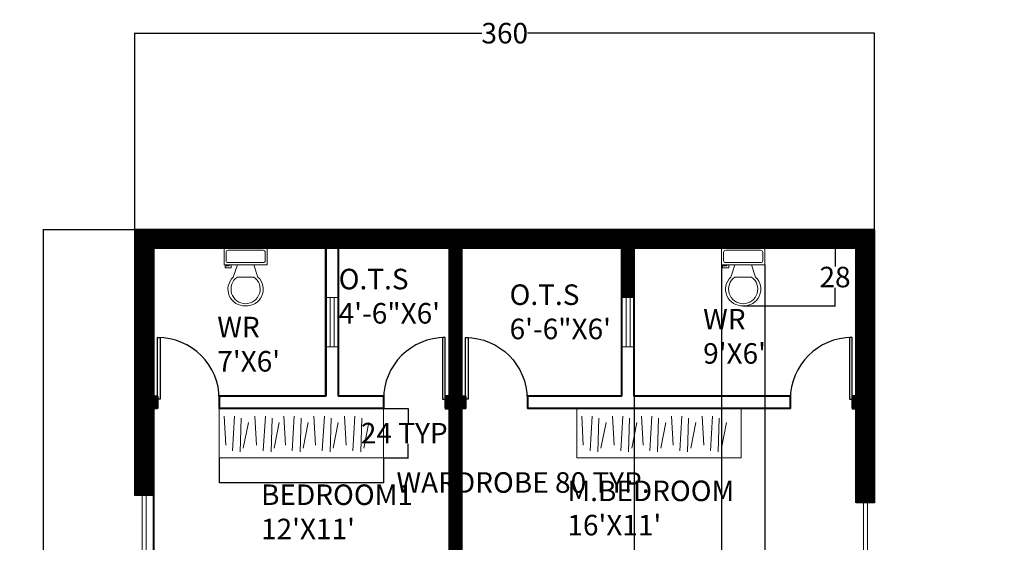
# Model space of a CAD drawing. Units: inches. Extents: x 345 to 1363, y 285 to 1014.
# Tile 2 of 4: x 345 to 824, y 760 to 1014. Entities that reach past the tile are written whole.
import ezdxf

# ---------------------------------------------------------------- set-up
doc = ezdxf.new("R2010")
doc.units = ezdxf.units.IN
doc.header["$MEASUREMENT"] = 0
for name, color, linetype, lineweight in [('A-ANNO-DIMS', 2, 'Continuous', 18), ('A-AREA-IDEN', 7, 'Continuous', 18), ('A-FLOR-CASE', 8, 'Continuous', 18), ('A-FLOR-FIXT', 9, 'Continuous', 18), ('A-GLAZ', 4, 'Continuous', 18), ('A-WALL', 7, 'Continuous', 40), ('A-WALL-PATT', 252, 'Continuous', 9), ('DOOR', 4, 'Continuous', 25)]:
    doc.layers.add(name, color=color, linetype=linetype, lineweight=lineweight)
doc.styles.get("Standard").update_dxf_attribs({"font": 'arial.ttf'})
doc.dimstyles.get("Standard").update_dxf_attribs({"dimtxt": 10, "dimasz": 0.18, "dimexe": 0.18, "dimexo": 0.0625, "dimgap": 0.09, "dimtad": 0, "dimtih": 1, "dimtoh": 1, "dimdec": 0, "dimzin": 0, "dimdsep": 46, "dimlunit": 3, "dimtxsty": 'Standard', "dimcen": 0.09, "dimadec": 0, "dimazin": 0, "dimtfac": 1, "dimtdec": 0, "dimtofl": 0, "dimtmove": 0, "dimatfit": 3, "dimfxl": 1, "dimtolj": 1, "dimtzin": 0, "dimarcsym": 0})

# ---------------------------------------------------------------- blocks, each defined once
blk = doc.blocks.new('*U4')
for p, q in [((0, 0), (0, -6)), ((40, 0), (40, -6))]:
    blk.add_line(p, q)
blk.add_lwpolyline([(0, 0), (0, 40), (1.75, 40), (1.75, 0)], close=True)
blk.add_arc((0, 0), 40, 0, 90)
blk = doc.blocks.new('*U8')
for p, q in [((0, 0), (0, -6)), ((-40, 0), (-40, -6))]:
    blk.add_line(p, q)
blk.add_lwpolyline([(0, 0), (0, 40), (-1.75, 40), (-1.75, 0)], close=True)
blk.add_arc((0, 0), 40, 90, 180)
blk = doc.blocks.new('*U6')
for p, q in [((9.5, -6), (9.5, -2)), ((-10, -8.5), (-8, -8.5)), ((-10, -9.5), (-10, -8.5)), ((-7, -9.5), (-10, -9.5)), ((-8, -8.5), (-8, -8)), ((-7, -8), (-7, -9.5)), ((-4, -8), (-6, -14)), ((4, -8), (6, -14)), ((4, -14), (-4, -14))]:
    blk.add_line(p, q)
blk.add_lwpolyline([(10.5, -8), (10.5, 0), (-10.5, 0), (-10.5, -8)], close=True)
for points in [[(-9.5, -2), (-9.5, -6)], [(8.5, -1), (-8.5, -1)], [(-8.5, -7), (8.5, -7)]]:
    blk.add_lwpolyline(points)
for centre, radius, start, end in [((-8.625, -1.875), 0.8839, 81.8699, 188.1301), ((8.625, -1.875), 0.8839, 351.8699, 98.1301), ((-8.625, -6.125), 0.8839, 171.869898, 278.1301), ((8.625, -6.125), 0.8839, 261.8699, 8.1301), ((-0.4772, -19.9188), 8.0953, 133.01722, 273.38), ((0.0374, -19.8731), 7.127, 124.50543, 269.7), ((-0.0373, -19.8731), 7.127, 270.3, 55.4946), ((0.4773, -19.9188), 8.0953, 266.62, 46.9828)]:
    blk.add_arc(centre, radius, start, end)
blk = doc.blocks.new('WIN-48IN-EXT')
for p, q in [((9, 48), (0, 48)), ((3.5, 0), (3.5, 48)), ((5.5, 0), (5.5, 48)), ((9, 0), (0, 0))]:
    blk.add_line(p, q)
blk = doc.blocks.new('WIN-24IN-VENT')
for p, q in [((0, 24), (6, 24)), ((2, 24), (2, 0)), ((4, 24), (4, 0)), ((0, 0), (6, 0))]:
    blk.add_line(p, q)
blk = doc.blocks.new('WARDROBE-80X24')
for p, q in [((0, 0), (0, 24)), ((80, 0), (80, 24)), ((2.45, 20.28), (3.21, 6.18)), ((7.49, 20.28), (6.48, 3.41)), ((10.77, 19.28), (10.26, 2.91)), ((17.45, 20.28), (18.2, 6.18)), ((22.49, 20.28), (21.48, 3.41)), ((25.77, 19.28), (25.26, 2.91)), ((31.55, 20.28), (32.31, 6.18)), ((36.59, 20.28), (35.59, 3.41)), ((39.87, 19.28), (39.37, 2.91)), ((46.16, 20.28), (46.91, 6.18)), ((51.2, 20.28), (50.19, 3.41)), ((54.47, 19.28), (53.97, 2.91)), ((61.07, 20.28), (61.83, 6.18)), ((66.11, 20.28), (65.1, 3.41)), ((69.39, 19.28), (68.88, 2.91)), ((14.3, 17.26), (11.77, 4.67)), ((29.29, 17.26), (26.77, 4.67)), ((43.4, 17.26), (40.88, 4.67)), ((58, 17.26), (55.48, 4.67)), ((72.92, 17.26), (70.4, 4.67)), ((80, 0), (0, 0))]:
    blk.add_line(p, q)
blk = doc.blocks.new('*D22')
at = {"layer": 'A-ANNO-DIMS', "color": 0, "lineweight": -2, "transparency": 16777216}
for p, q in [((441.97, 800.7), (441.97, 788.58)), ((521.97, 800.7), (521.97, 788.58)), ((442.15, 788.76), (521.79, 788.76)), ((521.97, 788.76), (522.15, 788.76))]:
    blk.add_line(p, q, dxfattribs=at)
at = {"layer": 'A-ANNO-DIMS', "color": 0, "transparency": 16777216}
for points in [[(442.15, 788.79), (442.15, 788.73), (441.97, 788.76)], [(521.79, 788.79), (521.79, 788.73), (521.97, 788.76)]]:
    blk.add_solid(points, dxfattribs=at)
at = {"layer": 'Defpoints', "color": 0, "transparency": 16777216}
for p in [(441.97, 800.76), (521.97, 800.76), (521.97, 788.76)]:
    blk.add_point(p, dxfattribs=at)
at = {"layer": 'A-ANNO-DIMS', "color": 0, "transparency": 16777216, "insert": (589.86, 788.76), "char_height": 10, "attachment_point": 5}
blk.add_mtext('\\A1;WARDROBE 80 TYP.', dxfattribs=at)
blk = doc.blocks.new('*D23')
at = {"layer": 'A-ANNO-DIMS', "color": 0, "lineweight": -2, "transparency": 16777216}
for p, q in [((522.03, 824.76), (534.15, 824.76)), ((533.97, 824.58), (533.97, 817.88)), ((533.97, 800.94), (533.97, 807.65)), ((522.03, 800.76), (534.15, 800.76))]:
    blk.add_line(p, q, dxfattribs=at)
at = {"layer": 'A-ANNO-DIMS', "color": 0, "transparency": 16777216}
for points in [[(533.94, 824.58), (534, 824.58), (533.97, 824.76)], [(533.94, 800.94), (534, 800.94), (533.97, 800.76)]]:
    blk.add_solid(points, dxfattribs=at)
at = {"layer": 'Defpoints', "color": 0, "transparency": 16777216}
for p in [(521.97, 824.76), (533.97, 824.76), (521.97, 800.76)]:
    blk.add_point(p, dxfattribs=at)
at = {"layer": 'A-ANNO-DIMS', "color": 0, "transparency": 16777216, "insert": (533.97, 812.76), "char_height": 10, "attachment_point": 5}
blk.add_mtext('\\A1;24 TYP.', dxfattribs=at)
blk = doc.blocks.new('*D30')
at = {"layer": 'A-ANNO-DIMS', "color": 0, "lineweight": -2, "transparency": 16777216}
for p, q in [((400.97, 911.83), (400.97, 1007.64)), ((401.15, 1007.46), (569.85, 1007.46)), ((760.79, 1007.46), (592.08, 1007.46)), ((760.97, 911.83), (760.97, 1007.64))]:
    blk.add_line(p, q, dxfattribs=at)
at = {"layer": 'A-ANNO-DIMS', "color": 0, "transparency": 16777216}
for points in [[(401.15, 1007.49), (401.15, 1007.43), (400.97, 1007.46)], [(760.79, 1007.49), (760.79, 1007.43), (760.97, 1007.46)]]:
    blk.add_solid(points, dxfattribs=at)
at = {"layer": 'Defpoints', "color": 0, "transparency": 16777216}
for p in [(760.97, 1007.46), (400.97, 911.76), (760.97, 911.76)]:
    blk.add_point(p, dxfattribs=at)
at = {"layer": 'A-ANNO-DIMS', "color": 0, "transparency": 16777216, "insert": (580.97, 1007.46), "char_height": 10, "attachment_point": 5}
blk.add_mtext('\\A1;360', dxfattribs=at)
blk = doc.blocks.new('*D31')
at = {"layer": 'A-ANNO-DIMS', "color": 0, "lineweight": -2, "transparency": 16777216}
for p, q in [((400.9, 911.76), (356.09, 911.76)), ((356.27, 911.58), (356.27, 628.96)), ((356.27, 335.94), (356.27, 618.57)), ((421.9, 335.76), (356.09, 335.76))]:
    blk.add_line(p, q, dxfattribs=at)
at = {"layer": 'A-ANNO-DIMS', "color": 0, "transparency": 16777216}
for points in [[(356.24, 911.58), (356.3, 911.58), (356.27, 911.76)], [(356.24, 335.94), (356.3, 335.94), (356.27, 335.76)]]:
    blk.add_solid(points, dxfattribs=at)
at = {"layer": 'Defpoints', "color": 0, "transparency": 16777216}
for p in [(356.27, 911.76), (400.97, 911.76), (421.97, 335.76)]:
    blk.add_point(p, dxfattribs=at)
at = {"layer": 'A-ANNO-DIMS', "color": 0, "transparency": 16777216, "insert": (356.27, 623.76), "char_height": 10, "attachment_point": 5}
blk.add_mtext('\\A1;576', dxfattribs=at)
blk = doc.blocks.new('*D43')
at = {"layer": 'A-ANNO-DIMS', "color": 0, "lineweight": -2, "transparency": 16777216}
for p, q in [((643.97, 902.7), (643.97, 290.88)), ((686.49, 894.7), (686.49, 290.88)), ((644.15, 291.06), (648.11, 291.06)), ((686.31, 291.06), (682.34, 291.06))]:
    blk.add_line(p, q, dxfattribs=at)
at = {"layer": 'A-ANNO-DIMS', "color": 0, "transparency": 16777216}
for points in [[(644.15, 291.09), (644.15, 291.03), (643.97, 291.06)], [(686.31, 291.09), (686.31, 291.03), (686.49, 291.06)]]:
    blk.add_solid(points, dxfattribs=at)
at = {"layer": 'Defpoints', "color": 0, "transparency": 16777216}
for p in [(643.97, 902.76), (686.49, 894.76), (686.49, 291.06)]:
    blk.add_point(p, dxfattribs=at)
at = {"layer": 'A-ANNO-DIMS', "color": 0, "transparency": 16777216, "insert": (665.23, 291.06), "char_height": 10, "attachment_point": 5}
blk.add_mtext('\\A1;42.52', dxfattribs=at)
blk = doc.blocks.new('*D44')
at = {"layer": 'A-ANNO-DIMS', "color": 0, "lineweight": -2, "transparency": 16777216}
for p, q in [((686.49, 894.7), (686.49, 290.88)), ((707.49, 894.7), (707.49, 290.88)), ((686.67, 291.06), (690.61, 291.06)), ((707.31, 291.06), (703.36, 291.06))]:
    blk.add_line(p, q, dxfattribs=at)
at = {"layer": 'A-ANNO-DIMS', "color": 0, "transparency": 16777216}
for points in [[(686.67, 291.09), (686.67, 291.03), (686.49, 291.06)], [(707.31, 291.09), (707.31, 291.03), (707.49, 291.06)]]:
    blk.add_solid(points, dxfattribs=at)
at = {"layer": 'Defpoints', "color": 0, "transparency": 16777216}
for p in [(686.49, 894.76), (707.49, 894.76), (707.49, 291.06)]:
    blk.add_point(p, dxfattribs=at)
at = {"layer": 'A-ANNO-DIMS', "color": 0, "transparency": 16777216, "insert": (696.99, 291.06), "char_height": 10, "attachment_point": 5}
blk.add_mtext('\\A1;21', dxfattribs=at)
blk = doc.blocks.new('*D45')
at = {"layer": 'A-ANNO-DIMS', "color": 0, "lineweight": -2, "transparency": 16777216}
for p, q in [((697.05, 902.76), (741.87, 902.76)), ((741.69, 902.58), (741.69, 893.96)), ((741.69, 874.94), (741.69, 883.57)), ((697.05, 874.76), (741.87, 874.76))]:
    blk.add_line(p, q, dxfattribs=at)
at = {"layer": 'A-ANNO-DIMS', "color": 0, "transparency": 16777216}
for points in [[(741.72, 902.58), (741.66, 902.58), (741.69, 902.76)], [(741.72, 874.94), (741.66, 874.94), (741.69, 874.76)]]:
    blk.add_solid(points, dxfattribs=at)
at = {"layer": 'Defpoints', "color": 0, "transparency": 16777216}
for p in [(696.99, 902.76), (696.99, 874.76), (741.69, 874.76)]:
    blk.add_point(p, dxfattribs=at)
at = {"layer": 'A-ANNO-DIMS', "color": 0, "transparency": 16777216, "insert": (741.69, 888.76), "char_height": 10, "attachment_point": 5}
blk.add_mtext('\\A1;28', dxfattribs=at)

msp = doc.modelspace()

# ---------------------------------------------------------------- hatches: boundary and pattern name
at = {"layer": 'A-WALL-PATT'}
h = msp.add_hatch(dxfattribs=at)
h.set_pattern_fill('ANSI31', color=256)
h.paths.add_polyline_path([(760.967, 730.806), (751.967, 730.806), (751.967, 692.764), (671.967, 692.764), (598.143, 692.764), (598.143, 686.764), (697.967, 686.764), (697.967, 586.835), (702.4, 586.835, -0.0130342), (703.967, 586.794), (703.967, 686.764), (751.967, 686.764), (751.967, 626.764), (742.74, 626.764), (742.74, 620.764), (751.967, 620.764), (751.967, 554.764), (703.967, 554.764), (703.967, 556.764), (702.4, 556.764), (697.967, 556.764), (697.967, 554.764), (622.228, 554.764), (622.228, 548.764), (751.967, 548.764), (751.967, 479.508), (760.967, 479.508)])
h.paths.add_polyline_path([(760.967, 431.508), (751.967, 431.508), (751.967, 380.764), (583.967, 380.764), (583.967, 548.764), (585.967, 548.764), (585.967, 549.325), (585.967, 554.764), (583.967, 554.764), (577.967, 554.764), (575.967, 554.764), (575.967, 548.764), (577.967, 548.764), (577.967, 371.764), (760.967, 371.764)])
h.paths.add_polyline_path([(409.967, 548.764), (529.967, 548.764), (529.967, 554.764), (511.967, 554.764), (511.967, 654.693), (507.456, 654.693, -0.0123881), (505.967, 654.73), (505.967, 554.764), (409.967, 554.764), (409.967, 596.764), (400.967, 596.764), (400.967, 371.764), (409.967, 371.764)])
h.paths.add_polyline_path([(409.967, 686.764), (505.967, 686.764), (505.967, 684.764), (507.456, 684.764), (511.967, 684.764), (511.967, 686.764), (515.791, 686.764), (515.791, 692.764), (409.967, 692.764), (409.967, 734.364), (400.967, 734.364), (400.967, 644.764), (409.967, 644.764)])
h.paths.add_polyline_path([(559.967, 824.764), (561.801, 824.764), (561.801, 829.275), (561.801, 830.764), (559.967, 830.764), (559.967, 902.764), (637.967, 902.764), (637.967, 878.764), (643.967, 878.764), (643.967, 902.764), (751.967, 902.764), (751.967, 830.764), (749.967, 830.764), (749.967, 829.275), (749.967, 824.764), (751.967, 824.764), (751.967, 778.806), (760.967, 778.806), (760.967, 911.764), (400.967, 911.764), (400.967, 782.364), (409.967, 782.364), (409.967, 824.764), (411.967, 824.764), (411.967, 829.275), (411.967, 830.764), (409.967, 830.764), (409.967, 902.764), (553.967, 902.764), (553.967, 830.764), (552.038, 830.764), (552.038, 829.275), (552.038, 824.764), (553.967, 824.764), (553.967, 692.764), (552.052, 692.764), (552.052, 692.203), (552.052, 686.764), (553.967, 686.764), (559.967, 686.764), (561.882, 686.764), (561.882, 692.764), (559.967, 692.764)])
h.paths.add_polyline_path([(718.74, 626.764), (703.967, 626.764), (703.967, 620.764), (718.74, 620.764)], flags=17)
h.paths.add_polyline_path([(892.382, 824.764), (894.382, 824.764), (894.382, 829.275), (894.382, 830.764), (892.382, 830.764), (892.382, 902.764), (1036.382, 902.764), (1036.382, 830.764), (1034.453, 830.764), (1034.453, 829.275), (1034.453, 824.764), (1036.382, 824.764), (1036.382, 692.764), (1034.467, 692.764), (1034.467, 692.203), (1034.467, 686.764), (1036.382, 686.764), (1042.382, 686.764), (1044.297, 686.764), (1044.297, 692.764), (1042.382, 692.764), (1042.382, 824.764), (1044.216, 824.764), (1044.216, 829.275), (1044.216, 830.764), (1042.382, 830.764), (1042.382, 902.764), (1120.382, 902.764), (1120.382, 878.764), (1126.382, 878.764), (1126.382, 902.764), (1234.382, 902.764), (1234.382, 830.764), (1232.382, 830.764), (1232.382, 829.275), (1232.382, 824.764), (1234.382, 824.764), (1234.382, 778.806), (1243.382, 778.806), (1243.382, 911.764), (883.382, 911.764), (883.382, 782.364), (892.382, 782.364)])
h.paths.add_polyline_path([(1243.382, 730.806), (1234.382, 730.806), (1234.382, 692.764), (1080.382, 692.764), (1080.382, 686.764), (1180.382, 686.764), (1180.382, 586.764), (1186.382, 586.764), (1186.382, 686.764), (1234.382, 686.764), (1234.382, 626.764), (1225.155, 626.764), (1225.155, 620.764), (1234.382, 620.764), (1234.382, 554.764), (1186.382, 554.764), (1186.382, 556.764), (1180.382, 556.764), (1180.382, 554.764), (1104.382, 554.764), (1104.382, 548.764), (1234.382, 548.764), (1234.382, 479.508), (1243.382, 479.508)])
h.paths.add_polyline_path([(892.382, 686.764), (988.382, 686.764), (988.382, 684.764), (989.871, 684.764), (994.382, 684.764), (994.382, 686.764), (998.206, 686.764), (998.206, 692.203, -0.0038664), (998.21, 692.764), (892.382, 692.764), (892.382, 734.364), (883.382, 734.364), (883.382, 644.764), (892.382, 644.764)])
h.paths.add_polyline_path([(1066.382, 548.764), (1068.382, 548.764), (1068.382, 554.764), (1066.382, 554.764), (1060.382, 554.764), (1058.382, 554.764), (1058.382, 548.764), (1060.382, 548.764), (1060.382, 371.764), (1243.382, 371.764), (1243.382, 431.508), (1234.382, 431.508), (1234.382, 380.764), (1154.382, 380.764), (1066.382, 380.764)])
h.paths.add_polyline_path([(1201.155, 626.764), (1186.382, 626.764), (1186.382, 620.764), (1201.155, 620.764)], flags=17)
h.paths.add_polyline_path([(892.382, 596.764), (883.382, 596.764), (883.382, 371.764), (892.382, 371.764), (892.382, 548.764), (1012.382, 548.764), (1012.382, 554.764), (994.382, 554.764), (994.382, 654.764), (988.382, 654.764), (988.382, 554.764), (892.382, 554.764)])

# ---------------------------------------------------------------- linework, layer by layer
at = {"layer": 'A-WALL'}
for p, q in [((760.967, 911.764), (400.967, 911.764)), ((400.967, 911.764), (400.967, 782.364)), ((760.967, 778.806), (760.967, 911.764)), ((409.967, 902.764), (409.967, 830.764)), ((553.967, 902.764), (409.967, 902.764)), ((493.967, 902.764), (493.967, 830.764)), ((493.967, 830.764), (493.967, 902.764)), ((499.967, 902.764), (499.967, 830.764)), ((553.967, 902.764), (553.967, 830.764)), ((559.967, 902.764), (559.967, 830.764)), ((637.967, 902.764), (559.967, 902.764)), ((637.967, 830.764), (637.967, 902.764)), ((751.967, 902.764), (643.967, 902.764)), ((643.967, 830.764), (643.967, 902.764)), ((751.967, 830.764), (751.967, 902.764)), ((409.967, 830.764), (411.967, 830.764)), ((411.967, 830.764), (411.967, 824.764)), ((441.967, 830.764), (441.967, 824.764)), ((493.967, 830.764), (441.967, 830.764)), ((521.967, 830.764), (499.967, 830.764)), ((521.967, 830.764), (521.967, 824.764)), ((553.967, 830.764), (551.967, 830.764)), ((551.967, 830.764), (551.967, 824.764)), ((559.967, 830.764), (561.967, 830.764)), ((561.801, 830.764), (561.801, 824.764)), ((591.967, 830.764), (591.967, 824.764)), ((637.967, 830.764), (591.967, 830.764)), ((719.967, 830.764), (643.967, 830.764)), ((719.967, 824.764), (719.967, 830.764)), ((751.967, 830.764), (749.967, 830.764)), ((749.967, 830.764), (749.967, 824.764)), ((411.967, 824.764), (409.967, 824.764)), ((409.967, 824.764), (409.967, 692.764)), ((521.967, 824.764), (441.967, 824.764)), ((551.967, 824.764), (553.967, 824.764)), ((553.967, 824.764), (553.967, 692.764)), ((561.967, 824.764), (559.967, 824.764)), ((559.967, 824.764), (559.967, 692.764)), ((719.967, 824.764), (591.967, 824.764)), ((749.967, 824.764), (751.967, 824.764)), ((751.967, 778.806), (751.967, 824.764))]:
    msp.add_line(p, q, dxfattribs=at)

# ---------------------------------------------------------------- block references
at = {"layer": 'A-FLOR-CASE'}
for p in [(441.967, 800.764), (615.967, 800.764)]:
    msp.add_blockref('WARDROBE-80X24', p, dxfattribs=at)
at = {"layer": 'A-FLOR-FIXT'}
for p in [(454.84, 902.764), (696.986, 902.764)]:
    msp.add_blockref('*U6', p, dxfattribs=at)
at = {"layer": 'A-GLAZ'}
for name, p in [('WIN-24IN-VENT', (493.967, 854.764)), ('WIN-48IN-EXT', (400.967, 734.364)), ('WIN-48IN-EXT', (751.967, 730.806))]:
    msp.add_blockref(name, p, dxfattribs=at)
at = {"layer": 'A-GLAZ', "rotation": 180}
msp.add_blockref('WIN-24IN-VENT', (643.967, 878.764), dxfattribs=at)
at = {"layer": 'DOOR', "yscale": 0.7517678943473934, "zscale": 0.7517678943473934}
for name, p, xscale in [('*U4', (411.967, 829.275), 0.7517678943473934), ('*U8', (552.038, 829.275), 0.7517678943473934), ('*U8', (561.801, 829.275), -0.7517678943473934), ('*U8', (749.967, 829.275), 0.7517678943473934)]:
    msp.add_blockref(name, p, dxfattribs=dict(at, xscale=xscale))

# ---------------------------------------------------------------- texts
at = {"layer": 'A-AREA-IDEN', "char_height": 10, "attachment_point": 1}
for s, insert in [('O.T.S\\P4\'-6"X6\'', (500.147, 892.783)), ('O.T.S\\P6\'-6"X6\'', (583.314, 885.171)), ("WR\\P9'X6'", (677.52, 873.248)), ("WR\\P7'X6'", (441.083, 869.418)), ("BEDROOM1\\P12'X11'", (462.36, 787.808)), ("M.BEDROOM\\P16'X11'", (611.44, 789.691))]:
    msp.add_mtext_dynamic_manual_height_columns(s, width=177.75817, gutter_width=1, heights=[0], dxfattribs=dict(at, insert=insert))

# ---------------------------------------------------------------- dimensions: what is measured, and where the dimension line sits
at = {"layer": 'A-ANNO-DIMS'}
for base, p1, p2, override, picture, middle in [((760.967, 1007.464), (400.967, 911.764), (760.967, 911.764), {"dimdec": 0, "dimlfac": 1, "dimrnd": 0, "dimzin": 0, "dimdsep": 46, "dimlunit": 2}, '*D30', (580.967, 1007.464)), ((686.486, 291.064), (643.967, 902.764), (686.486, 894.764), {"dimdec": 2, "dimlfac": 1, "dimrnd": 0, "dimzin": 0, "dimdsep": 46, "dimlunit": 2}, '*D43', (665.226, 291.064)), ((707.486, 291.064), (686.486, 894.764), (707.486, 894.764), {"dimdec": 0, "dimlfac": 1, "dimrnd": 0, "dimzin": 0, "dimdsep": 46, "dimlunit": 2}, '*D44', (696.986, 291.064))]:
    dim = msp.add_linear_dim(base=base, p1=p1, p2=p2, dimstyle='Standard', override=override, dxfattribs=at)
    dim.commit()
    dim.dimension.update_dxf_attribs({"geometry": picture, "text_midpoint": middle})
for base, p1, p2, angle, picture, middle in [((356.267, 911.764), (421.967, 335.764), (400.967, 911.764), 90, '*D31', (356.267, 623.764)), ((741.686, 874.764), (696.986, 902.764), (696.986, 874.764), 270.00016, '*D45', (741.686, 888.764))]:
    dim = msp.add_linear_dim(base=base, p1=p1, p2=p2, angle=angle, dimstyle='Standard', override={"dimdec": 0, "dimlfac": 1, "dimrnd": 0, "dimzin": 0, "dimdsep": 46, "dimlunit": 2}, dxfattribs=at)
    dim.commit()
    dim.dimension.update_dxf_attribs({"geometry": picture, "text_midpoint": middle})
dim = msp.add_linear_dim(base=(533.967, 824.764), p1=(521.967, 800.764), p2=(521.967, 824.764), angle=90, text='<> TYP.', dimstyle='Standard', override={"dimdec": 0, "dimlfac": 1, "dimrnd": 0, "dimzin": 0, "dimdsep": 46, "dimlunit": 2}, dxfattribs=at)
dim.commit()
dim.dimension.update_dxf_attribs({"geometry": '*D23', "text_midpoint": (533.967, 812.764)})
dim = msp.add_linear_dim(base=(521.967, 788.764), p1=(441.967, 800.764), p2=(521.967, 800.764), text='WARDROBE <> TYP.', dimstyle='Standard', override={"dimdec": 0, "dimlfac": 1, "dimrnd": 0, "dimzin": 0, "dimdsep": 46, "dimlunit": 2}, dxfattribs=at)
dim.commit()
dim.dimension.update_dxf_attribs({"geometry": '*D22', "text_midpoint": (589.856, 788.764)})

doc.saveas('drawing.dxf')
